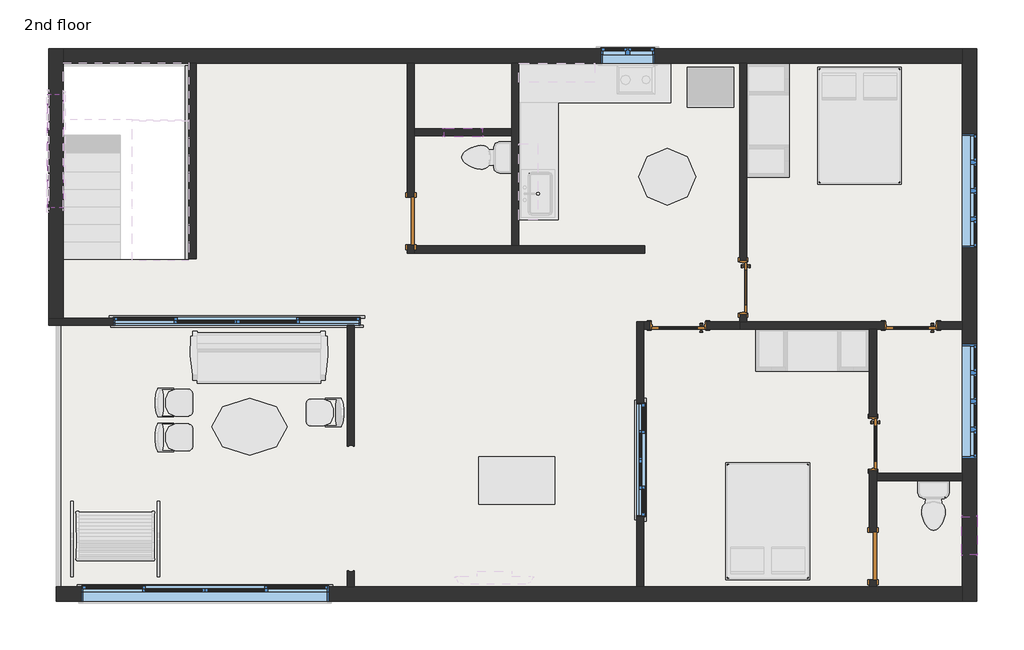
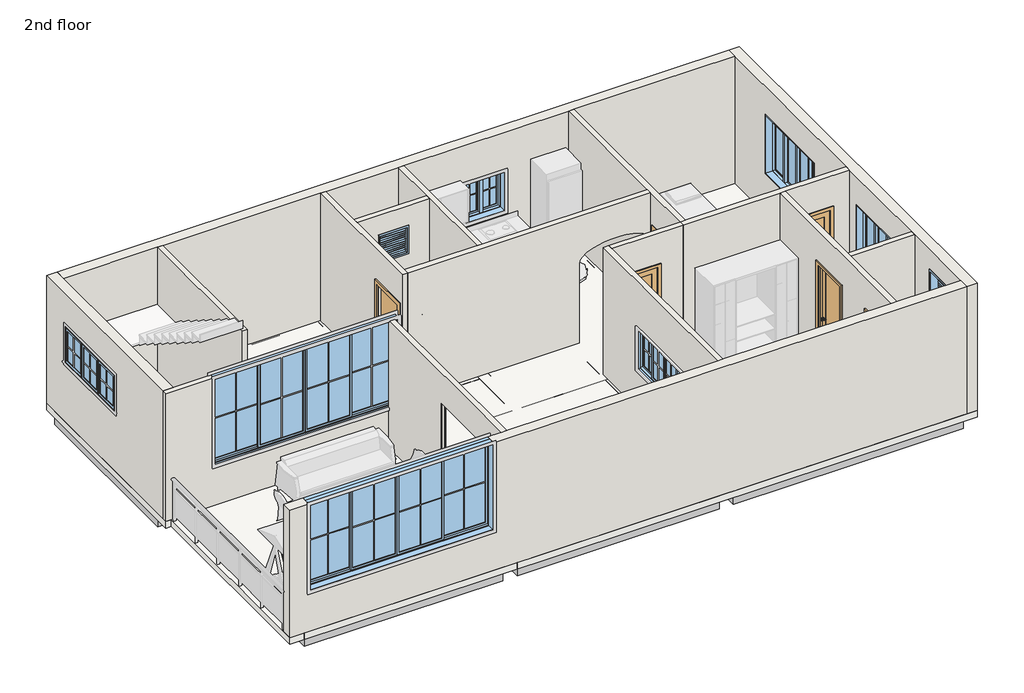
# One storey, part 1 of 2: 17 walls, 9 beams, 9 windows, 6 doors, 1 slab.
# Revit data of these elements (continued)
# Element 35 (IfcWindow, "Window-Casement-Double : 34\" x 36\"") (continued)
#   Frame Extension = 0.020833 ft
#   Exterior Wall Closure = 0.104167 ft
#   Interior Trim Visibility = yes
#   Exterior Trim Visibility = yes
#   Phase Created = New Construction
#   Materials on its faces: "Wood - Stained", "Glass", "Clad - White"
# Element 36 (IfcWindow, "Window-Casement-Multi-Sash-Horizontal : 72\" x 53\"")
#   Mark = "21"
#   Window Inset = 0.052083 ft
#   Frame Gap 3 = 0.13737 ft
#   Frame Gap 2 = 0.052083 ft
#   Phase Created = New Construction
#   Materials on its faces: "Metal - Aluminum", "Glass"
# Element 37 (IfcWindow, "Window-Casement-Multi-Sash-Horizontal : 72\" x 53\"")
#   Mark = "24"
#   Window Inset = 0.052083 ft
#   Frame Gap 3 = 0.13737 ft
#   Frame Gap 2 = 0.052083 ft
#   Phase Created = New Construction
#   Materials on its faces: "Metal - Aluminum", "Glass"
# Element 38 (IfcWindow, "Window-Louvers : 24\" x 24\"")
#   Mark = "22"
#   Blade Width = 1.875 ft
#   Phase Created = New Construction
#   Materials on its faces: "Birch"
# Element 39 (IfcWindow, "Window-Louvers : 24\" x 24\"")
#   Mark = "23"
#   Blade Width = 1.875 ft
#   Phase Created = New Construction
#   Materials on its faces: "Birch"
# Element 40 (IfcWindow, "Window-Sliding-Four : 156\" x 78\"")
#   Mark = "19"
#   Window Inset = 0 ft
#   Interior Wall Closure = 0.216146 ft
#   Frame Extension = 0.020833 ft
#   Exterior Wall Closure = 0.104167 ft
#   Interior Trim Visibility = yes
#   Indicator Visibility = yes
#   Exterior Trim Visibility = yes
#   Phase Created = New Construction
#   Materials on its faces: "Wood - Stained", "Glass", "Clad - White"
# Element 41 (IfcWindow, "Window-Sliding-Four : 156\" x 78\"")
#   Mark = "29"
#   Window Inset = 0 ft
#   Interior Wall Closure = 0.216146 ft
#   Frame Extension = 0.020833 ft
#   Exterior Wall Closure = 0.104167 ft
#   Interior Trim Visibility = yes
#   Indicator Visibility = yes
#   Exterior Trim Visibility = yes
#   Phase Created = New Construction
#   Materials on its faces: "Wood - Stained", "Glass", "Clad - White"
# Element 42 (IfcWindow, "Window-Sliding-Four : 72\" x 36\"")
#   Mark = "20"
#   Window Inset = 0 ft
#   Interior Wall Closure = 0.216146 ft
#   Frame Extension = 0.020833 ft
#   Exterior Wall Closure = 0.104167 ft
#   Interior Trim Visibility = yes
#   Indicator Visibility = yes
#   Exterior Trim Visibility = yes
#   Phase Created = New Construction
#   Materials on its faces: "Wood - Stained", "Glass", "Clad - White"
# Materials
#   "Concrete, Cast-in-Place gray": class "Concrete", colour RGB 192 192 192, transparency 0, Description = "Cast-in-place concrete", Cost = 0
#   "Cherry": class "Wood", colour RGB 226 177 128, transparency 0, Description = "Prunus Serotina", Cost = 0
#   "Aluminum": class "Metal", colour RGB 247 247 247, transparency 0, Description = "Aluminum 6061", Cost = 0
#   "Door - Panel": class "Wood", colour RGB 210 159 95, transparency 0, Cost = 0
#   "Door - Frame": colour RGB 118 70 51, transparency 0, Cost = 0
#   "Wood - Stained": class "Wood", colour RGB 224 178 126, transparency 0, Cost = 0
#   "Glass": class "Glass", colour RGB 0 128 192, transparency 0.75, Description = "Soda Lime Glass", Cost = 0
#   "Clad - White": class "Wood", colour RGB 242 242 238, transparency 0, Cost = 0
#   "Metal - Aluminum": class "Metal", colour RGB 247 247 247, transparency 0
#   "Birch": class "Wood", colour RGB 224 178 126, transparency 0, Description = "Betula Alleghaniensis", Cost = 0
#   "Default Floor": colour RGB 128 128 128, transparency 0, Cost = 0
#   "Default Wall": colour RGB 128 128 128, transparency 0, Cost = 0
